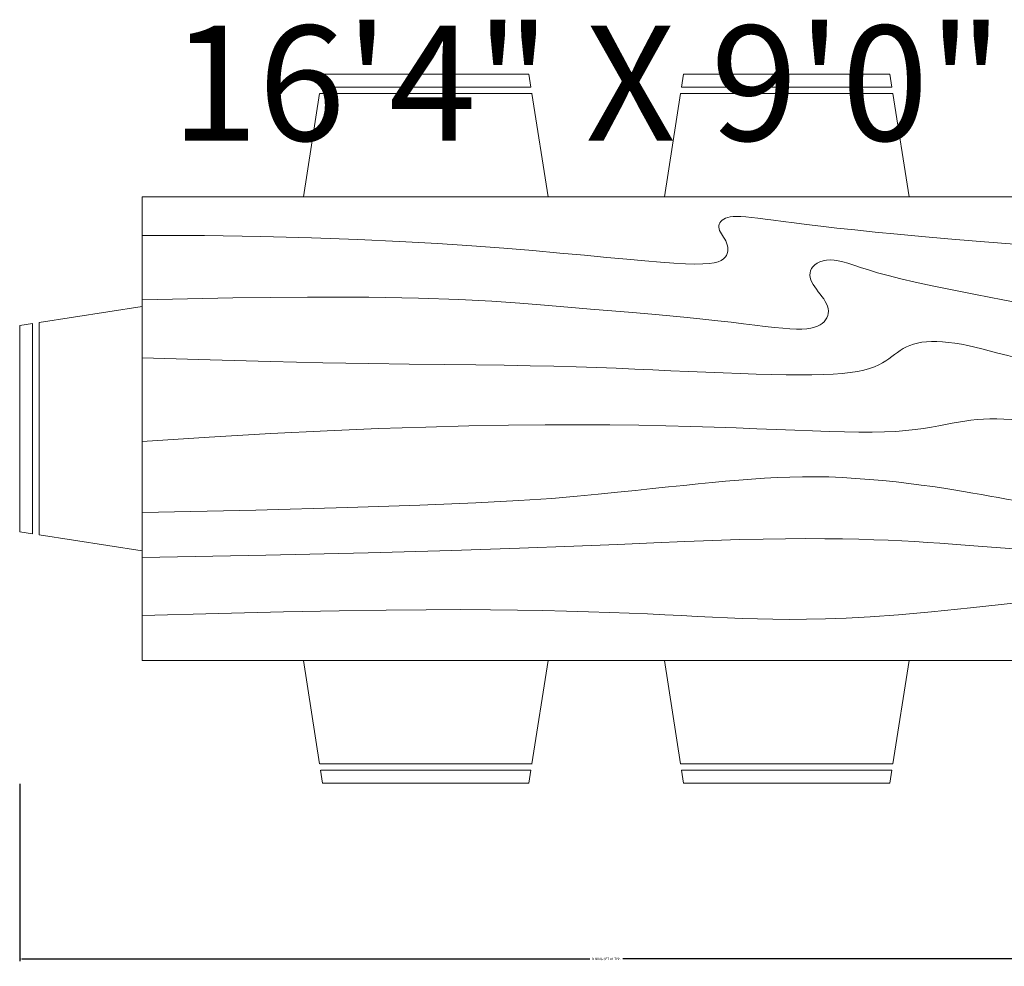
# Model space of a CAD drawing. Units: inches. Extents: x -46 to 1145, y -527 to 760.
# Tile 46 of 57: x 212 to 288, y 395 to 469. Entities that reach past the tile are written whole.
import ezdxf

# ---------------------------------------------------------------- set-up
doc = ezdxf.new("R2010")
doc.units = ezdxf.units.IN
doc.header["$MEASUREMENT"] = 0
for name, color, linetype, lineweight in [('A-ANNO-DIMS', 2, 'Continuous', 18), ('A-AREA-IDEN', 1, 'Continuous', 18), ('A-FURN', 2, 'Continuous', 13)]:
    doc.layers.add(name, color=color, linetype=linetype, lineweight=lineweight)
doc.styles.get("Standard").update_dxf_attribs({"font": 'arial.ttf'})
doc.dimstyles.get("Standard").update_dxf_attribs({"dimtxt": 0.18, "dimasz": 0.18, "dimexe": 0.18, "dimexo": 0.0625, "dimgap": 0.09, "dimtad": 0, "dimtih": 1, "dimtoh": 1, "dimdec": 0, "dimzin": 0, "dimdsep": 46, "dimlunit": 3, "dimtxsty": 'Standard', "dimcen": 0.09, "dimadec": 0, "dimazin": 0, "dimtfac": 1, "dimtdec": 0, "dimtofl": 0, "dimtmove": 0, "dimatfit": 3, "dimfxl": 1, "dimtolj": 1, "dimtzin": 0, "dimarcsym": 0})

# ---------------------------------------------------------------- blocks, each defined once
blk = doc.blocks.new('Dining Set - 36 x 72 in.')
for p, q in [((-22, 27.5), (-22.1562, 26.50042)), ((-22, 27.5), (-6, 27.5)), ((-5.8437, 26.49966), (-6, 27.5)), ((6, 27.5), (5.8438, 26.50042)), ((6, 27.5), (22, 27.5)), ((22.1563, 26.49966), (22, 27.5)), ((-22.2343, 26.00059), (-23.4847, 17.99762)), ((-22.2304, 26), (-5.7608, 26)), ((-5.8416, 26.5), (-22.1534, 26.5)), ((-4.5152, 17.99762), (-5.7655, 25.99926)), ((5.7657, 26.00059), (4.5153, 17.99762)), ((5.7696, 26), (22.2392, 26)), ((22.1584, 26.5), (5.8466, 26.5)), ((23.4848, 17.99762), (22.2345, 25.99926)), ((36, 18), (-36, 18)), ((-36, 18), (-36, -18)), ((36, -18), (36, 18)), ((-44.0006, 8.23428), (-35.9976, 9.48474)), ((44.0006, 8.23428), (35.9976, 9.48474)), ((-45.5, 8), (-44.5004, 8.15617)), ((-45.5, 8), (-45.5, -8)), ((-44.5, -8.15843), (-44.5, 8.15338)), ((-44, 8.23041), (-44, -8.23915)), ((44, 8.23041), (44, -8.23915)), ((44.5, -8.15843), (44.5, 8.15338)), ((45.5, 8), (44.5005, 8.15617)), ((45.5, 8), (45.5, -8)), ((-44.4997, -8.15631), (-45.5, -8)), ((-35.9976, -9.48476), (-43.9993, -8.2345)), ((35.9976, -9.48476), (43.9993, -8.2345)), ((44.4997, -8.15631), (45.5, -8)), ((-36, -18), (36, -18)), ((-22.2343, -26.0006), (-23.4847, -17.99762)), ((-4.5152, -17.99762), (-5.7655, -25.99928)), ((5.7657, -26.0006), (4.5153, -17.99762)), ((23.4848, -17.99762), (22.2345, -25.99928)), ((-22.2304, -26), (-5.7608, -26)), ((-22, -27.5), (-22.1562, -26.50044)), ((-5.8416, -26.5), (-22.1534, -26.5)), ((-5.8437, -26.49967), (-6, -27.5)), ((5.7696, -26), (22.2392, -26)), ((6, -27.5), (5.8438, -26.50044)), ((22.1584, -26.5), (5.8466, -26.5)), ((22.1563, -26.49967), (22, -27.5)), ((-22, -27.5), (-6, -27.5)), ((6, -27.5), (22, -27.5))]:
    blk.add_line(p, q)
for points in [[(-36, 15), (-31.1772, 14.97754), (-26.8079, 14.91406), (-22.8538, 14.81543), (-19.276, 14.6875), (-16.0362, 14.53613), (-13.0957, 14.36718), (-10.4159, 14.18652), (-7.9583, 14), (-5.6904, 13.81315), (-3.6035, 13.63021), (-1.6954, 13.45508), (0.0365, 13.29166), (1.5945, 13.14388), (2.9811, 13.01562), (4.1988, 12.9108), (5.25, 12.83333), (6.1393, 12.78613), (6.8802, 12.76823), (7.4883, 12.77767), (7.9792, 12.8125), (8.3685, 12.87077), (8.6719, 12.95052), (8.9049, 13.0498), (9.0833, 13.16666), (9.2205, 13.29899), (9.3216, 13.44401), (9.3895, 13.59879), (9.4271, 13.76041), (9.4373, 13.92594), (9.4232, 14.09245), (9.3875, 14.257), (9.3333, 14.41666), (9.2638, 14.56917), (9.1836, 14.71484), (9.0975, 14.85465), (9.0104, 14.98958), (8.9272, 15.1206), (8.8529, 15.2487), (8.7922, 15.37483), (8.75, 15.5), (8.7305, 15.62467), (8.7344, 15.74739), (8.7617, 15.86621), (8.8125, 15.97916), (8.8867, 16.08431), (8.9844, 16.17968), (9.1055, 16.26334), (9.25, 16.33333), (9.4189, 16.38802), (9.6172, 16.42708), (9.8506, 16.45052), (10.125, 16.45833), (10.4463, 16.45052), (10.8203, 16.42708), (11.2529, 16.38802), (11.75, 16.33333), (12.3184, 16.26318), (12.9694, 16.17838), (13.7151, 16.07991), (14.5677, 15.96875), (15.5395, 15.84586), (16.6426, 15.71224), (17.8893, 15.56884), (19.2917, 15.41666), (20.859, 15.25667), (22.5879, 15.08984), (24.4721, 14.91715), (26.5052, 14.73958), (28.6809, 14.5581), (30.9929, 14.3737), (33.4347, 14.18733), (36, 14)], [(-36, 10), (-28.9766, 10.14274), (-23.1725, 10.20442), (-18.4241, 10.19775), (-14.5677, 10.13541), (-11.4399, 10.03011), (-8.877, 9.89453), (-6.7154, 9.74137), (-4.7917, 9.58333), (-2.9698, 9.43082), (-1.2246, 9.28515), (0.4415, 9.14534), (2.026, 9.01041), (3.5266, 8.87939), (4.9408, 8.7513), (6.266, 8.62516), (7.5, 8.5), (8.6411, 8.37549), (9.6914, 8.2539), (10.6538, 8.13818), (11.5312, 8.03125), (12.3267, 7.93603), (13.043, 7.85547), (13.6831, 7.79248), (14.25, 7.75), (14.7471, 7.7303), (15.1797, 7.73307), (15.5537, 7.75732), (15.875, 7.80208), (16.1494, 7.86637), (16.3828, 7.94922), (16.5811, 8.04964), (16.75, 8.16666), (16.8944, 8.29915), (17.0143, 8.44531), (17.1089, 8.60319), (17.1771, 8.77083), (17.218, 8.94629), (17.2305, 9.1276), (17.2137, 9.31282), (17.1667, 9.5), (17.0895, 9.6875), (16.987, 9.875), (16.8649, 10.0625), (16.7292, 10.25), (16.5856, 10.4375), (16.4401, 10.625), (16.2985, 10.8125), (16.1667, 11), (16.05, 11.18733), (15.9518, 11.3737), (15.8752, 11.5581), (15.8229, 11.73958), (15.798, 11.91715), (15.8034, 12.08984), (15.842, 12.25667), (15.9167, 12.41666), (16.0295, 12.56836), (16.1784, 12.70833), (16.3605, 12.83268), (16.5729, 12.9375), (16.8127, 13.01888), (17.0768, 13.07291), (17.3625, 13.0957), (17.6667, 13.08333), (17.9894, 13.03312), (18.3418, 12.94726), (18.7382, 12.82918), (19.1927, 12.68229), (19.7195, 12.51001), (20.3327, 12.31575), (21.0465, 12.10294), (21.875, 11.875), (22.8357, 11.63354), (23.959, 11.37304), (25.2786, 11.08618), (26.8282, 10.76562), (28.6414, 10.40405), (30.752, 9.99414), (33.1936, 9.52856), (36, 9)], [(-36, 5.5), (-30.7157, 5.3348), (-26.069, 5.20963), (-21.9946, 5.11767), (-18.4271, 5.05208), (-15.3009, 5.00602), (-12.5508, 4.97265), (-10.1112, 4.94515), (-7.9167, 4.91666), (-5.909, 4.88167), (-4.0586, 4.83984), (-2.3429, 4.79215), (-0.7396, 4.73958), (0.7739, 4.6831), (2.22, 4.6237), (3.6213, 4.56233), (5, 4.5), (6.373, 4.43782), (7.7344, 4.3776), (9.0723, 4.32129), (10.375, 4.27083), (11.6309, 4.22819), (12.8281, 4.19531), (13.9551, 4.17415), (15, 4.16666), (15.954, 4.17448), (16.819, 4.19791), (17.6001, 4.23698), (18.3021, 4.29166), (18.9299, 4.36198), (19.4883, 4.44791), (19.9823, 4.54948), (20.4167, 4.66666), (20.7969, 4.79899), (21.1302, 4.94401), (21.4245, 5.09879), (21.6875, 5.26041), (21.9271, 5.42594), (22.1511, 5.59245), (22.3672, 5.757), (22.5834, 5.91666), (22.8065, 6.06868), (23.0404, 6.21093), (23.2879, 6.34147), (23.5521, 6.45833), (23.8358, 6.55957), (24.142, 6.64323), (24.4735, 6.70735), (24.8334, 6.75), (25.2235, 6.76969), (25.642, 6.76692), (26.0858, 6.74267), (26.5521, 6.69791), (27.0379, 6.63362), (27.5404, 6.55078), (28.0565, 6.45036), (28.5834, 6.33333), (29.1242, 6.19987), (29.7071, 6.04687), (30.3661, 5.87044), (31.1354, 5.66666), (32.0493, 5.43164), (33.142, 5.16146), (34.4475, 4.85221), (36, 4.5)], [(-36, -1), (-30.7915, -0.6591), (-26.0195, -0.38216), (-21.6519, -0.16284), (-17.6563, 0.00521), (-14.0005, 0.12833), (-10.6523, 0.21289), (-7.5796, 0.26522), (-4.75, 0.29166), (-2.134, 0.29793), (0.2878, 0.28711), (2.5317, 0.26163), (4.6146, 0.22396), (6.5529, 0.17651), (8.3633, 0.12174), (10.0623, 0.06209), (11.6667, 0), (13.1899, -0.06201), (14.6341, -0.1211), (15.9982, -0.17432), (17.2813, -0.21875), (18.4823, -0.25147), (19.6003, -0.26953), (20.6343, -0.27002), (21.5834, -0.25), (22.4481, -0.20768), (23.2357, -0.14584), (23.9549, -0.06836), (24.6146, 0.02083), (25.2235, 0.11784), (25.7904, 0.21875), (26.3241, 0.31966), (26.8334, 0.41666), (27.3265, 0.50618), (27.8099, 0.58593), (28.2894, 0.65397), (28.7709, 0.70833), (29.2601, 0.74707), (29.763, 0.76823), (30.2855, 0.76985), (30.8334, 0.75), (31.4088, 0.70784), (31.9994, 0.64713), (32.589, 0.57275), (33.1615, 0.48958), (33.7008, 0.4025), (34.1908, 0.3164), (34.6153, 0.23616), (34.9584, 0.16666), (35.2099, 0.11165), (35.3848, 0.07031), (35.504, 0.04069), (35.5886, 0.02083), (35.6594, 0.00879), (35.7377, 0.0026), (35.8442, 0.00032), (36, 0)], [(-36, -6.5), (-27.1843, -6.31267), (-20.084, -6.1263), (-14.469, -5.9419), (-10.1094, -5.76042), (-6.7752, -5.58285), (-4.2363, -5.41016), (-2.2629, -5.24333), (-0.625, -5.08334), (0.8708, -4.93099), (2.2715, -4.78646), (3.5872, -4.64974), (4.8281, -4.52084), (6.0046, -4.39974), (7.127, -4.28646), (8.2053, -4.18099), (9.25, -4.08334), (10.2705, -3.99382), (11.2734, -3.91407), (12.2647, -3.84603), (13.25, -3.79167), (14.2354, -3.75293), (15.2266, -3.73177), (16.2295, -3.73015), (17.25, -3.75), (18.2912, -3.79248), (19.3451, -3.85547), (20.4009, -3.93604), (21.4479, -4.03125), (22.4754, -4.13819), (23.4727, -4.25391), (24.4289, -4.37549), (25.3334, -4.5), (26.1785, -4.62492), (26.9694, -4.74935), (27.7145, -4.87281), (28.4219, -4.99479), (29.1, -5.11483), (29.7572, -5.23242), (30.4016, -5.34709), (31.0417, -5.45834), (31.6837, -5.56437), (32.3262, -5.65821), (32.9658, -5.73153), (33.599, -5.77604), (34.2224, -5.78345), (34.8327, -5.74545), (35.4264, -5.65373), (36, -5.5)], [(-36, -10), (-26.4022, -9.81299), (-18.4675, -9.62891), (-11.9839, -9.45069), (-6.7396, -9.28125), (-2.5226, -9.12354), (0.8789, -8.98047), (3.6769, -8.85498), (6.0833, -8.75), (8.2767, -8.66765), (10.3021, -8.60677), (12.1712, -8.56543), (13.8958, -8.54167), (15.4876, -8.53353), (16.9583, -8.53907), (18.3197, -8.55632), (19.5834, -8.58334), (20.7616, -8.61841), (21.8685, -8.66081), (22.9188, -8.71004), (23.9271, -8.76563), (24.9081, -8.82707), (25.8763, -8.89388), (26.8465, -8.96558), (27.8334, -9.04167), (28.8474, -9.12118), (29.8828, -9.20117), (30.93, -9.27824), (31.9792, -9.34896), (33.0205, -9.40991), (34.0443, -9.45768), (35.0407, -9.48885), (36, -9.5)], [(-36, -14.5), (-30.0881, -14.33513), (-25.0332, -14.21224), (-20.7312, -14.12647), (-17.0781, -14.07292), (-13.97, -14.04671), (-11.3027, -14.04297), (-8.9724, -14.05681), (-6.875, -14.08334), (-4.9224, -14.11833), (-3.0905, -14.16016), (-1.3709, -14.20785), (0.2448, -14.26042), (1.7647, -14.3169), (3.1973, -14.3763), (4.5507, -14.43767), (5.8333, -14.5), (7.0554, -14.5621), (8.235, -14.62175), (9.3922, -14.67652), (10.5469, -14.72396), (11.7192, -14.76164), (12.929, -14.78711), (14.1965, -14.79794), (15.5417, -14.79167), (16.9933, -14.76424), (18.6152, -14.70508), (20.4804, -14.60197), (22.6615, -14.44271), (25.2312, -14.21509), (28.2624, -13.9069), (31.8277, -13.50594), (36, -13)]]:
    blk.add_lwpolyline(points)
blk = doc.blocks.new('*D676')
at = {"layer": 'A-ANNO-DIMS', "color": 0, "lineweight": -2, "transparency": 16777216}
for p, q in [((211.862, 409.395), (211.862, 395.627)), ((302.862, 409.395), (302.862, 395.627)), ((212.042, 395.807), (256.084, 395.807)), ((302.682, 395.807), (258.64, 395.807))]:
    blk.add_line(p, q, dxfattribs=at)
at = {"layer": 'A-ANNO-DIMS', "color": 0, "transparency": 16777216}
for points in [[(212.042, 395.837), (212.042, 395.777), (211.862, 395.807)], [(302.682, 395.837), (302.682, 395.777), (302.862, 395.807)]]:
    blk.add_solid(points, dxfattribs=at)
at = {"layer": 'Defpoints', "color": 0, "transparency": 16777216}
for p in [(211.862, 409.457), (302.862, 409.457), (302.862, 395.807)]:
    blk.add_point(p, dxfattribs=at)
at = {"layer": 'A-ANNO-DIMS', "color": 0, "transparency": 16777216, "insert": (257.362, 395.807), "char_height": 0.18, "attachment_point": 5}
blk.add_mtext('\\A1;DINING SET 91 TYP.', dxfattribs=at)

msp = doc.modelspace()

# ---------------------------------------------------------------- block references
at = {"layer": 'A-FURN'}
msp.add_blockref('Dining Set - 36 x 72 in.', (257.3617, 436.9572), dxfattribs=at)

# ---------------------------------------------------------------- texts
at = {"layer": 'A-AREA-IDEN'}
msp.add_text('16\'4" X 9\'0"', height=8.923264, dxfattribs=at).set_placement((223.6059, 459.3065))

# ---------------------------------------------------------------- dimensions: what is measured, and where the dimension line sits
at = {"layer": 'A-ANNO-DIMS'}
dim = msp.add_linear_dim(base=(302.8617, 395.8072), p1=(211.8617, 409.4572), p2=(302.8617, 409.4572), text='DINING SET <> TYP.', dimstyle='Standard', override={"dimdec": 0, "dimlfac": 1, "dimrnd": 0, "dimzin": 0, "dimdsep": 46, "dimlunit": 2}, dxfattribs=at)
dim.commit()
dim.dimension.update_dxf_attribs({"geometry": '*D676', "text_midpoint": (257.3617, 395.8072)})

doc.saveas('drawing.dxf')
